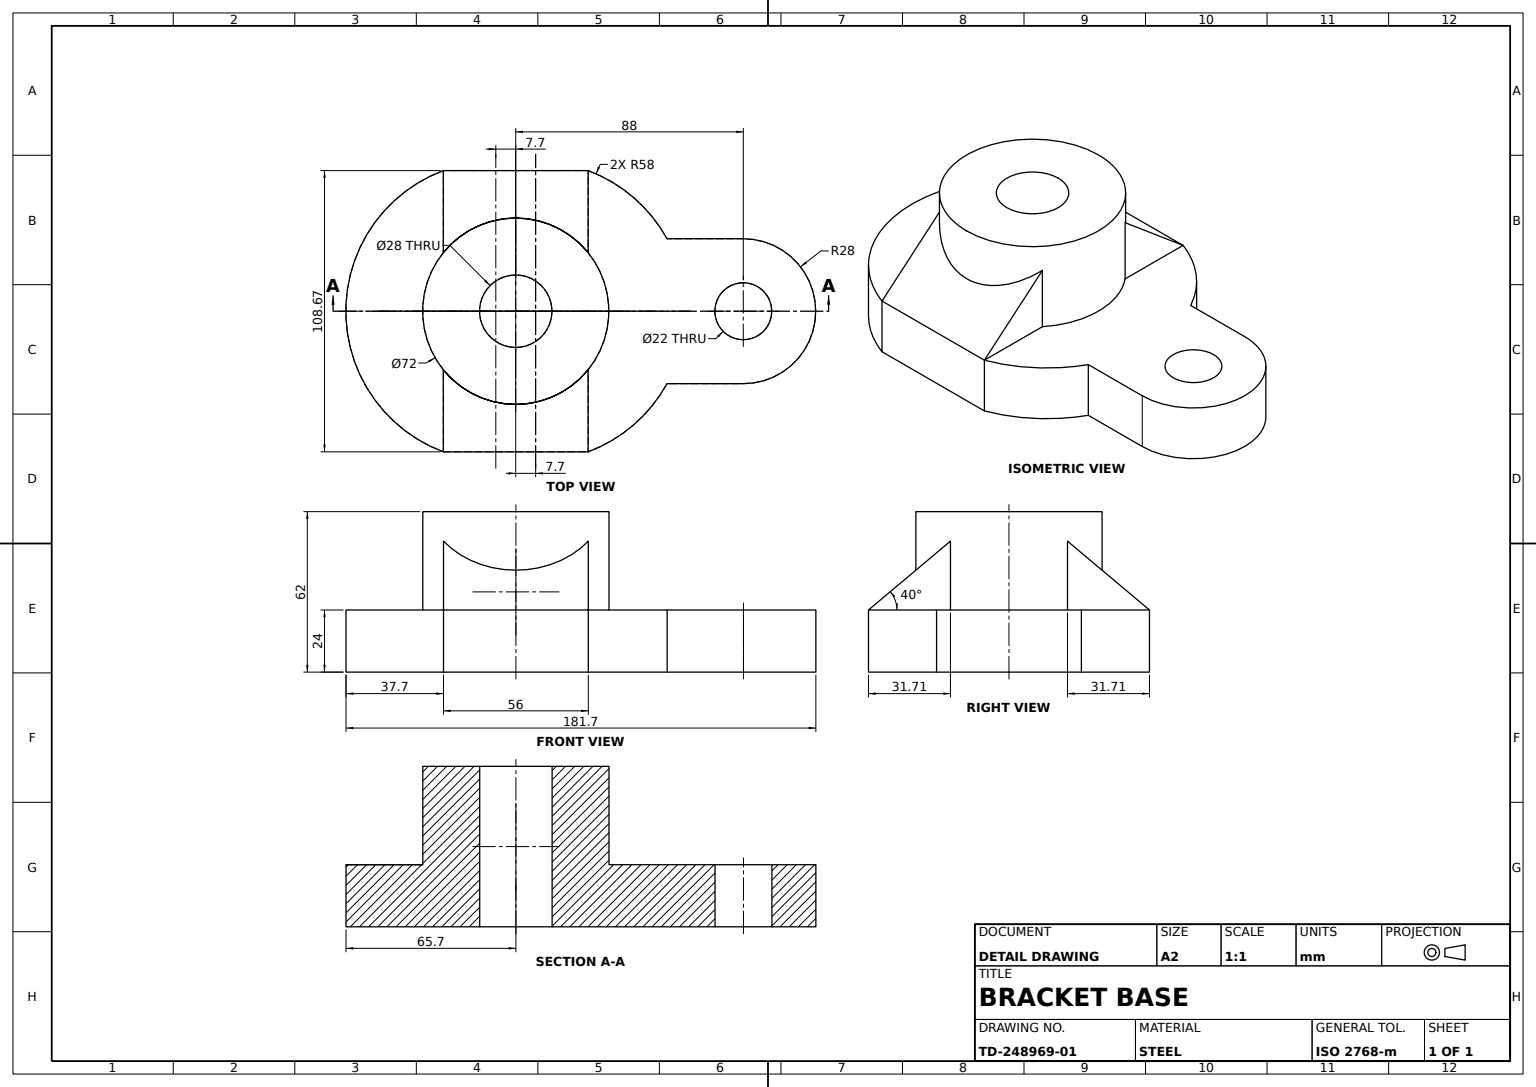
from build123d import *

# Parameters (mm, degrees)
BASE_FLANGE_SKETCH_R = 11
BASE_FLANGE_DEPTH    = 24
HUB_BOSS_SKETCH_72_R = 36
HUB_BOSS_72_DEPTH    = 38
WEDGE_SUPPORT_DEPTH  = 28
BORE_28_REACH        = 176.416
BORE_SKETCH_28_R     = 14


with BuildPart() as part:
    # Base Flange Sketch → Base Flange (new body)
    with BuildSketch(Plane(origin=(0, 0, 0), x_dir=(1, 0, 0), z_dir=(0, 1, 0))):
        with BuildLine():
            Line((-116, 54.332778116), (-60, 54.332778116))
            ThreePointArc((-60, 54.332778116), (-42.391267518, 43.899782505), (-29.502831874, 28))
            Line((-29.502831874, 28), (0, 28))
            ThreePointArc((0, 28), (28, 0), (0, -28))
            Line((0, -28), (-29.502831874, -28))
            ThreePointArc((-29.502831874, -28), (-42.391267518, -43.899782505), (-60, -54.332778116))
            Line((-60, -54.332778116), (-116, -54.332778116))
            ThreePointArc((-116, -54.332778116), (-153.703467729, 0), (-116, 54.332778116))
        make_face()
        with Locations(Location((0, 0, 0), (0, 0, 270))):
            Circle(BASE_FLANGE_SKETCH_R, mode=Mode.SUBTRACT)
    extrude(amount=BASE_FLANGE_DEPTH)

    # Hub Boss Sketch Ø72 → Hub Boss Ø72 (add)
    with BuildSketch(Plane(origin=(0, 24, 0), x_dir=(1, 0, 0), z_dir=(0, 1, 0))):
        with Locations(Location((-88, 0, 0), (0, 0, 270))):
            Circle(HUB_BOSS_SKETCH_72_R)
    extrude(amount=HUB_BOSS_72_DEPTH)

    # Wedge Support Sketch → Wedge Support (add, symmetric)
    with BuildSketch(Plane(origin=(-88, 0, 0), x_dir=(0, 0, -1), z_dir=(1, 0, 0))):
        Polygon((-54.332778116, 24), (-13.504322415, 58.25914212), (13.266446181, 58.45874398), (54.332778116, 24), align=None)
    extrude(amount=WEDGE_SUPPORT_DEPTH, both=True)

    # Bore Sketch Ø28 → Bore Ø28 (cut, up to next)
    with BuildSketch(Plane(origin=(0, 62, 0), x_dir=(1, 0, 0), z_dir=(0, 1, 0)), mode=Mode.PRIVATE) as bore_28_sk1:
        with Locations(Location((-88, 0, 0), (0, 0, 270))):
            Circle(BORE_SKETCH_28_R)
    bore_28_tool1 = extrude(bore_28_sk1.sketch, amount=-BORE_28_REACH, mode=Mode.PRIVATE) & part.part
    add(bore_28_tool1.solids().sort_by_distance((-88, 62, 0))[0], mode=Mode.SUBTRACT)


solid = part.part
